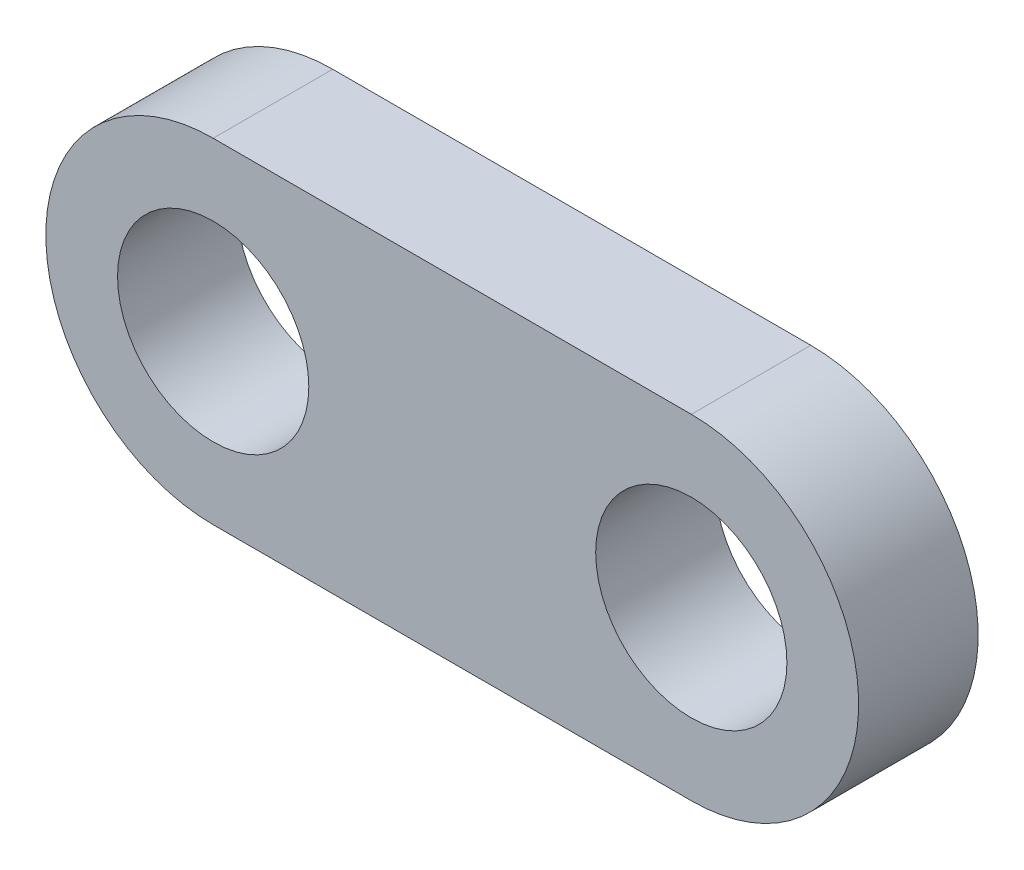
ISO-10303-21;
HEADER;
FILE_DESCRIPTION(('STEP AP214'),'2;1');
FILE_NAME('part.step','',(''),(''),'','','');
FILE_SCHEMA(('AUTOMOTIVE_DESIGN { 1 0 10303 214 1 1 1 1 }'));
ENDSEC;
DATA;
#1=APPLICATION_CONTEXT('core data for automotive mechanical design processes');
#2=APPLICATION_PROTOCOL_DEFINITION('international standard','automotive_design',2000,#1);
#3=PRODUCT_CONTEXT('',#1,'mechanical');
#4=PRODUCT('Part','Part','',(#3));
#5=PRODUCT_RELATED_PRODUCT_CATEGORY('part','',(#4));
#6=PRODUCT_DEFINITION_FORMATION('','',#4);
#7=PRODUCT_DEFINITION_CONTEXT('part definition',#1,'design');
#8=PRODUCT_DEFINITION('design','',#6,#7);
#9=PRODUCT_DEFINITION_SHAPE('','',#8);
#10=(LENGTH_UNIT() NAMED_UNIT(*) SI_UNIT(.MILLI.,.METRE.));
#11=(NAMED_UNIT(*) PLANE_ANGLE_UNIT() SI_UNIT($,.RADIAN.));
#12=(NAMED_UNIT(*) SI_UNIT($,.STERADIAN.) SOLID_ANGLE_UNIT());
#13=UNCERTAINTY_MEASURE_WITH_UNIT(LENGTH_MEASURE(1.E-05),#10,'distance_accuracy_value','');
#14=(GEOMETRIC_REPRESENTATION_CONTEXT(3) GLOBAL_UNCERTAINTY_ASSIGNED_CONTEXT((#13)) GLOBAL_UNIT_ASSIGNED_CONTEXT((#10,
#11,#12)) REPRESENTATION_CONTEXT('',''));
#15=CARTESIAN_POINT('',(0.,0.,0.));
#16=DIRECTION('',(0.,0.,1.));
#17=DIRECTION('',(1.,0.,0.));
#18=AXIS2_PLACEMENT_3D('',#15,#16,#17);
#19=CARTESIAN_POINT('',(-10.,0.,2.5));
#20=DIRECTION('',(0.,0.,1.));
#21=DIRECTION('',(1.,0.,0.));
#22=AXIS2_PLACEMENT_3D('',#19,#20,#21);
#23=PLANE('',#22);
#24=CARTESIAN_POINT('',(-10.,0.,2.5));
#25=DIRECTION('',(0.,0.,1.));
#26=DIRECTION('',(1.,0.,0.));
#27=AXIS2_PLACEMENT_3D('',#24,#25,#26);
#28=CIRCLE('',#27,4.);
#29=CARTESIAN_POINT('',(-6.,0.,2.5));
#30=VERTEX_POINT('',#29);
#31=EDGE_CURVE('E107',#30,#30,#28,.T.);
#32=ORIENTED_EDGE('',*,*,#31,.F.);
#33=EDGE_LOOP('',(#32));
#34=FACE_BOUND('',#33,.T.);
#35=CARTESIAN_POINT('',(-10.,0.,2.5));
#36=DIRECTION('',(0.,0.,1.));
#37=DIRECTION('',(1.,0.,0.));
#38=AXIS2_PLACEMENT_3D('',#35,#36,#37);
#39=CIRCLE('',#38,7.);
#40=CARTESIAN_POINT('',(-10.,7.,2.5));
#41=VERTEX_POINT('',#40);
#42=CARTESIAN_POINT('',(-10.,-7.,2.5));
#43=VERTEX_POINT('',#42);
#44=EDGE_CURVE('E91',#41,#43,#39,.T.);
#45=ORIENTED_EDGE('',*,*,#44,.T.);
#46=DIRECTION('',(1.,0.,0.));
#47=VECTOR('',#46,1.);
#48=CARTESIAN_POINT('',(-10.,-7.,2.5));
#49=LINE('',#48,#47);
#50=CARTESIAN_POINT('',(10.,-7.,2.5));
#51=VERTEX_POINT('',#50);
#52=EDGE_CURVE('E86',#43,#51,#49,.T.);
#53=ORIENTED_EDGE('',*,*,#52,.T.);
#54=CARTESIAN_POINT('',(10.,0.,2.5));
#55=DIRECTION('',(0.,0.,1.));
#56=DIRECTION('',(1.,0.,0.));
#57=AXIS2_PLACEMENT_3D('',#54,#55,#56);
#58=CIRCLE('',#57,7.);
#59=CARTESIAN_POINT('',(10.,7.,2.5));
#60=VERTEX_POINT('',#59);
#61=EDGE_CURVE('E93',#51,#60,#58,.T.);
#62=ORIENTED_EDGE('',*,*,#61,.T.);
#63=DIRECTION('',(-1.,0.,0.));
#64=VECTOR('',#63,1.);
#65=CARTESIAN_POINT('',(-10.,7.,2.5));
#66=LINE('',#65,#64);
#67=EDGE_CURVE('E59',#60,#41,#66,.T.);
#68=ORIENTED_EDGE('',*,*,#67,.T.);
#69=EDGE_LOOP('',(#45,#53,#62,#68));
#70=FACE_BOUND('',#69,.T.);
#71=CARTESIAN_POINT('',(10.,0.,2.5));
#72=DIRECTION('',(0.,0.,1.));
#73=DIRECTION('',(1.,0.,0.));
#74=AXIS2_PLACEMENT_3D('',#71,#72,#73);
#75=CIRCLE('',#74,4.);
#76=CARTESIAN_POINT('',(14.,0.,2.5));
#77=VERTEX_POINT('',#76);
#78=EDGE_CURVE('E123',#77,#77,#75,.T.);
#79=ORIENTED_EDGE('',*,*,#78,.F.);
#80=EDGE_LOOP('',(#79));
#81=FACE_BOUND('',#80,.T.);
#82=ADVANCED_FACE('F41',(#34,#70,#81),#23,.T.);
#83=CARTESIAN_POINT('',(-10.,0.,-2.5));
#84=DIRECTION('',(0.,0.,1.));
#85=DIRECTION('',(1.,0.,0.));
#86=AXIS2_PLACEMENT_3D('',#83,#84,#85);
#87=PLANE('',#86);
#88=CARTESIAN_POINT('',(-10.,0.,-2.5));
#89=DIRECTION('',(0.,0.,1.));
#90=DIRECTION('',(1.,0.,0.));
#91=AXIS2_PLACEMENT_3D('',#88,#89,#90);
#92=CIRCLE('',#91,7.);
#93=CARTESIAN_POINT('',(-10.,7.,-2.5));
#94=VERTEX_POINT('',#93);
#95=CARTESIAN_POINT('',(-10.,-7.,-2.5));
#96=VERTEX_POINT('',#95);
#97=EDGE_CURVE('E104',#94,#96,#92,.T.);
#98=ORIENTED_EDGE('',*,*,#97,.F.);
#99=DIRECTION('',(-1.,0.,0.));
#100=VECTOR('',#99,1.);
#101=CARTESIAN_POINT('',(-10.,7.,-2.5));
#102=LINE('',#101,#100);
#103=CARTESIAN_POINT('',(10.,7.,-2.5));
#104=VERTEX_POINT('',#103);
#105=EDGE_CURVE('E81',#104,#94,#102,.T.);
#106=ORIENTED_EDGE('',*,*,#105,.F.);
#107=CARTESIAN_POINT('',(10.,0.,-2.5));
#108=DIRECTION('',(0.,0.,1.));
#109=DIRECTION('',(1.,0.,0.));
#110=AXIS2_PLACEMENT_3D('',#107,#108,#109);
#111=CIRCLE('',#110,7.);
#112=CARTESIAN_POINT('',(10.,-7.,-2.5));
#113=VERTEX_POINT('',#112);
#114=EDGE_CURVE('E73',#113,#104,#111,.T.);
#115=ORIENTED_EDGE('',*,*,#114,.F.);
#116=DIRECTION('',(1.,0.,0.));
#117=VECTOR('',#116,1.);
#118=CARTESIAN_POINT('',(-10.,-7.,-2.5));
#119=LINE('',#118,#117);
#120=EDGE_CURVE('E100',#96,#113,#119,.T.);
#121=ORIENTED_EDGE('',*,*,#120,.F.);
#122=EDGE_LOOP('',(#98,#106,#115,#121));
#123=FACE_BOUND('',#122,.T.);
#124=CARTESIAN_POINT('',(-10.,0.,-2.5));
#125=DIRECTION('',(0.,0.,1.));
#126=DIRECTION('',(1.,0.,0.));
#127=AXIS2_PLACEMENT_3D('',#124,#125,#126);
#128=CIRCLE('',#127,4.);
#129=CARTESIAN_POINT('',(-6.,0.,-2.5));
#130=VERTEX_POINT('',#129);
#131=EDGE_CURVE('E118',#130,#130,#128,.T.);
#132=ORIENTED_EDGE('',*,*,#131,.T.);
#133=EDGE_LOOP('',(#132));
#134=FACE_BOUND('',#133,.T.);
#135=CARTESIAN_POINT('',(10.,0.,-2.5));
#136=DIRECTION('',(0.,0.,1.));
#137=DIRECTION('',(1.,0.,0.));
#138=AXIS2_PLACEMENT_3D('',#135,#136,#137);
#139=CIRCLE('',#138,4.);
#140=CARTESIAN_POINT('',(14.,0.,-2.5));
#141=VERTEX_POINT('',#140);
#142=EDGE_CURVE('E127',#141,#141,#139,.T.);
#143=ORIENTED_EDGE('',*,*,#142,.T.);
#144=EDGE_LOOP('',(#143));
#145=FACE_BOUND('',#144,.T.);
#146=ADVANCED_FACE('F117',(#123,#134,#145),#87,.F.);
#147=CARTESIAN_POINT('',(-10.,0.,2.5));
#148=DIRECTION('',(0.,0.,-1.));
#149=DIRECTION('',(-1.,0.,0.));
#150=AXIS2_PLACEMENT_3D('',#147,#148,#149);
#151=CYLINDRICAL_SURFACE('',#150,7.);
#152=ORIENTED_EDGE('',*,*,#97,.T.);
#153=DIRECTION('',(0.,0.,-1.));
#154=VECTOR('',#153,1.);
#155=CARTESIAN_POINT('',(-10.,-7.,2.5));
#156=LINE('',#155,#154);
#157=EDGE_CURVE('E11',#43,#96,#156,.T.);
#158=ORIENTED_EDGE('',*,*,#157,.F.);
#159=ORIENTED_EDGE('',*,*,#44,.F.);
#160=DIRECTION('',(0.,0.,-1.));
#161=VECTOR('',#160,1.);
#162=CARTESIAN_POINT('',(-10.,7.,2.5));
#163=LINE('',#162,#161);
#164=EDGE_CURVE('E101',#41,#94,#163,.T.);
#165=ORIENTED_EDGE('',*,*,#164,.T.);
#166=EDGE_LOOP('',(#152,#158,#159,#165));
#167=FACE_BOUND('',#166,.T.);
#168=ADVANCED_FACE('F43',(#167),#151,.T.);
#169=CARTESIAN_POINT('',(-10.,-7.,2.5));
#170=DIRECTION('',(0.,1.,0.));
#171=DIRECTION('',(-1.,0.,0.));
#172=AXIS2_PLACEMENT_3D('',#169,#170,#171);
#173=PLANE('',#172);
#174=ORIENTED_EDGE('',*,*,#120,.T.);
#175=DIRECTION('',(0.,0.,-1.));
#176=VECTOR('',#175,1.);
#177=CARTESIAN_POINT('',(10.,-7.,2.5));
#178=LINE('',#177,#176);
#179=EDGE_CURVE('E49',#51,#113,#178,.T.);
#180=ORIENTED_EDGE('',*,*,#179,.F.);
#181=ORIENTED_EDGE('',*,*,#52,.F.);
#182=ORIENTED_EDGE('',*,*,#157,.T.);
#183=EDGE_LOOP('',(#174,#180,#181,#182));
#184=FACE_BOUND('',#183,.T.);
#185=ADVANCED_FACE('F96',(#184),#173,.F.);
#186=CARTESIAN_POINT('',(10.,0.,2.5));
#187=DIRECTION('',(0.,0.,-1.));
#188=DIRECTION('',(-1.,0.,0.));
#189=AXIS2_PLACEMENT_3D('',#186,#187,#188);
#190=CYLINDRICAL_SURFACE('',#189,7.);
#191=ORIENTED_EDGE('',*,*,#114,.T.);
#192=DIRECTION('',(0.,0.,-1.));
#193=VECTOR('',#192,1.);
#194=CARTESIAN_POINT('',(10.,7.,2.5));
#195=LINE('',#194,#193);
#196=EDGE_CURVE('E98',#60,#104,#195,.T.);
#197=ORIENTED_EDGE('',*,*,#196,.F.);
#198=ORIENTED_EDGE('',*,*,#61,.F.);
#199=ORIENTED_EDGE('',*,*,#179,.T.);
#200=EDGE_LOOP('',(#191,#197,#198,#199));
#201=FACE_BOUND('',#200,.T.);
#202=ADVANCED_FACE('F97',(#201),#190,.T.);
#203=CARTESIAN_POINT('',(-10.,7.,2.5));
#204=DIRECTION('',(0.,-1.,0.));
#205=DIRECTION('',(1.,0.,0.));
#206=AXIS2_PLACEMENT_3D('',#203,#204,#205);
#207=PLANE('',#206);
#208=ORIENTED_EDGE('',*,*,#105,.T.);
#209=ORIENTED_EDGE('',*,*,#164,.F.);
#210=ORIENTED_EDGE('',*,*,#67,.F.);
#211=ORIENTED_EDGE('',*,*,#196,.T.);
#212=EDGE_LOOP('',(#208,#209,#210,#211));
#213=FACE_BOUND('',#212,.T.);
#214=ADVANCED_FACE('F114',(#213),#207,.F.);
#215=CARTESIAN_POINT('',(-10.,0.,2.5));
#216=DIRECTION('',(0.,0.,-1.));
#217=DIRECTION('',(-1.,0.,0.));
#218=AXIS2_PLACEMENT_3D('',#215,#216,#217);
#219=CYLINDRICAL_SURFACE('',#218,4.);
#220=ORIENTED_EDGE('',*,*,#31,.T.);
#221=EDGE_LOOP('',(#220));
#222=FACE_BOUND('',#221,.T.);
#223=ORIENTED_EDGE('',*,*,#131,.F.);
#224=EDGE_LOOP('',(#223));
#225=FACE_BOUND('',#224,.T.);
#226=ADVANCED_FACE('F141',(#222,#225),#219,.F.);
#227=CARTESIAN_POINT('',(10.,0.,2.5));
#228=DIRECTION('',(0.,0.,-1.));
#229=DIRECTION('',(-1.,0.,0.));
#230=AXIS2_PLACEMENT_3D('',#227,#228,#229);
#231=CYLINDRICAL_SURFACE('',#230,4.);
#232=ORIENTED_EDGE('',*,*,#78,.T.);
#233=EDGE_LOOP('',(#232));
#234=FACE_BOUND('',#233,.T.);
#235=ORIENTED_EDGE('',*,*,#142,.F.);
#236=EDGE_LOOP('',(#235));
#237=FACE_BOUND('',#236,.T.);
#238=ADVANCED_FACE('F135',(#234,#237),#231,.F.);
#239=CLOSED_SHELL('',(#82,#146,#168,#185,#202,#214,#226,#238));
#240=MANIFOLD_SOLID_BREP('B2',#239);
#241=ADVANCED_BREP_SHAPE_REPRESENTATION('',(#18,#240),#14);
#242=SHAPE_DEFINITION_REPRESENTATION(#9,#241);
ENDSEC;
END-ISO-10303-21;
